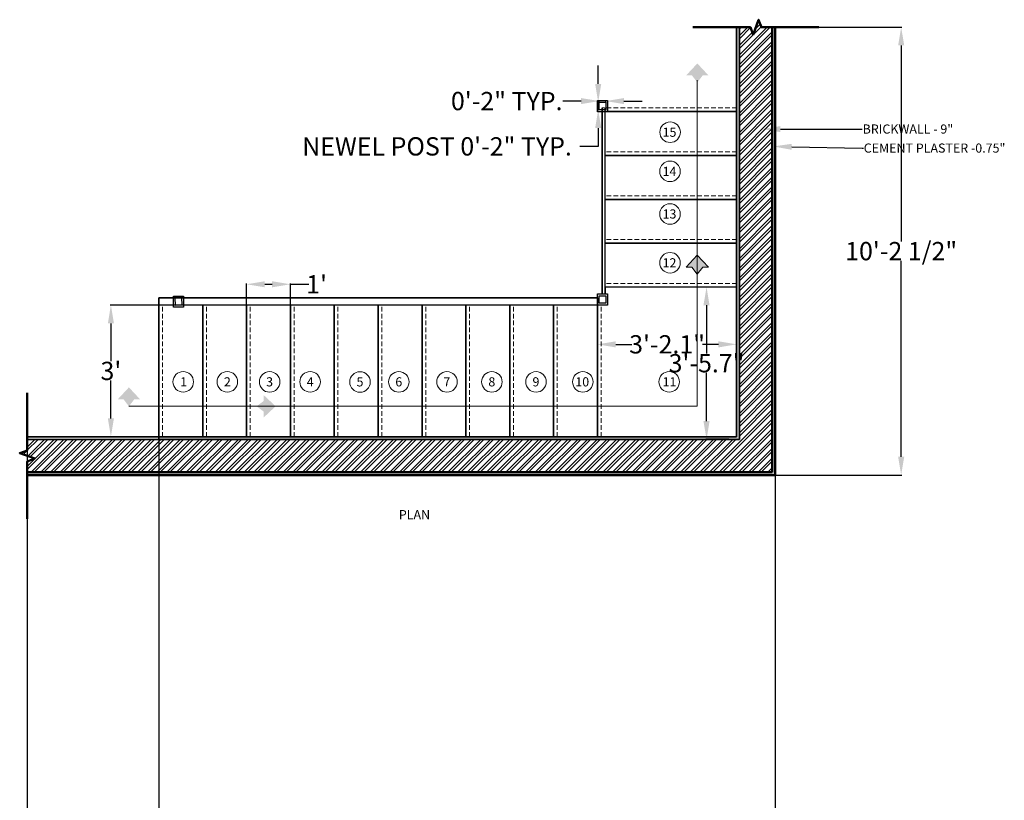
# Model space of a CAD drawing. Units: inches. Extents: x -17 to 288, y -625 to -149.
# Tile 2 of 2: x 18 to 288, y -363 to -149. Entities that reach past the tile are written whole.
import ezdxf
from ezdxf import colors
from ezdxf.entities.mleader import LeaderData, LeaderLine
from ezdxf.math import Vec2, Vec3

# ---------------------------------------------------------------- set-up
doc = ezdxf.new("R2010")
doc.units = ezdxf.units.IN
doc.header["$MEASUREMENT"] = 0
doc.linetypes.add('HIDDEN', pattern=[9.525, 6.35, -3.175])
for name, color, linetype, lineweight in [('A-ANNO-DIMS', 2, 'Continuous', 18), ('A-ANNO-SYMB', 3, 'Continuous', 18), ('A-ANNO-TEXT', 7, 'Continuous', 18), ('A-FLOR-HRAL', 4, 'Continuous', 25), ('A-FLOR-STRS', 1, 'Continuous', 35), ('A-FLOR-STRS-HIDN', 8, 'HIDDEN', 18), ('A-WALL', 7, 'Continuous', 50), ('A-WALL-PATT', 8, 'Continuous', 18)]:
    doc.layers.add(name, color=color, linetype=linetype, lineweight=lineweight)
doc.styles.get("Standard").update_dxf_attribs({"font": 'arial.ttf'})
doc.dimstyles.get("Standard").update_dxf_attribs({"dimtxt": 5, "dimasz": 5, "dimexe": 0.18, "dimexo": 0.0625, "dimgap": 0.09, "dimtad": 0, "dimtih": 1, "dimtoh": 1, "dimdec": 1, "dimzin": 0, "dimdsep": 46, "dimlunit": 3, "dimtxsty": 'Standard', "dimcen": 0, "dimadec": 0, "dimazin": 0, "dimtfac": 1, "dimtdec": 1, "dimtofl": 0, "dimtmove": 0, "dimatfit": 3, "dimfxl": 1, "dimtolj": 1, "dimtzin": 0, "dimarcsym": 1})

# ---------------------------------------------------------------- blocks, each defined once
blk = doc.blocks.new('*D2')
at = {"layer": 'A-ANNO-DIMS', "color": 0, "lineweight": -2, "transparency": 16777216}
for p, q in [((56.28, -227), (43.05, -227)), ((43.23, -232), (43.23, -242.35)), ((43.23, -258), (43.23, -247.64)), ((56.28, -263), (43.05, -263))]:
    blk.add_line(p, q, dxfattribs=at)
at = {"layer": 'A-ANNO-DIMS', "color": 0, "transparency": 16777216}
for points in [[(42.4, -232), (44.07, -232), (43.23, -227)], [(42.4, -258), (44.07, -258), (43.23, -263)]]:
    blk.add_solid(points, dxfattribs=at)
at = {"layer": 'Defpoints', "color": 0, "transparency": 16777216}
for p in [(56.34, -227), (43.23, -263), (56.34, -263)]:
    blk.add_point(p, dxfattribs=at)
at = {"layer": 'A-ANNO-DIMS', "color": 0, "transparency": 16777216, "insert": (43.23, -245), "char_height": 5, "attachment_point": 5}
blk.add_mtext("\\A1;3'", dxfattribs=at)
blk = doc.blocks.new('*D3')
at = {"layer": 'A-ANNO-DIMS', "color": 0, "lineweight": -2, "transparency": 16777216}
for p, q in [((80.34, -226.93), (80.34, -221.11)), ((85.34, -221.29), (87.34, -221.29)), ((92.34, -226.93), (92.34, -221.11)), ((92.34, -221.29), (97.34, -221.29))]:
    blk.add_line(p, q, dxfattribs=at)
at = {"layer": 'A-ANNO-DIMS', "color": 0, "transparency": 16777216}
for points in [[(85.34, -220.46), (85.34, -222.12), (80.34, -221.29)], [(87.34, -220.46), (87.34, -222.12), (92.34, -221.29)]]:
    blk.add_solid(points, dxfattribs=at)
at = {"layer": 'Defpoints', "color": 0, "transparency": 16777216}
for p in [(92.34, -221.29), (80.34, -227), (92.34, -227)]:
    blk.add_point(p, dxfattribs=at)
at = {"layer": 'A-ANNO-DIMS', "color": 0, "transparency": 16777216, "insert": (99.5, -221.29), "char_height": 5, "attachment_point": 5}
blk.add_mtext("\\A1;1'", dxfattribs=at)
blk = doc.blocks.new('*D5')
at = {"layer": 'A-ANNO-DIMS', "color": 0, "lineweight": -2, "transparency": 16777216}
for p, q in [((176.34, -237.39), (176.34, -237.91)), ((181.34, -237.73), (185.73, -237.73)), ((209.41, -237.73), (205.03, -237.73)), ((214.41, -237.39), (214.41, -237.91))]:
    blk.add_line(p, q, dxfattribs=at)
at = {"layer": 'A-ANNO-DIMS', "color": 0, "transparency": 16777216}
for points in [[(181.34, -236.9), (181.34, -238.57), (176.34, -237.73)], [(209.41, -236.9), (209.41, -238.57), (214.41, -237.73)]]:
    blk.add_solid(points, dxfattribs=at)
at = {"layer": 'Defpoints', "color": 0, "transparency": 16777216}
for p in [(176.34, -237.33), (214.41, -237.33), (214.41, -237.73)]:
    blk.add_point(p, dxfattribs=at)
at = {"layer": 'A-ANNO-DIMS', "color": 0, "transparency": 16777216, "insert": (195.38, -237.73), "char_height": 5, "attachment_point": 5}
blk.add_mtext('\\A1;3\'-2.1"', dxfattribs=at)
blk = doc.blocks.new('*D6')
at = {"layer": 'A-ANNO-DIMS', "color": 0, "lineweight": -2, "transparency": 16777216}
for p, q in [((211.19, -222.05), (205.99, -222.05)), ((206.17, -227.05), (206.17, -240.24)), ((206.17, -258.72), (206.17, -245.53)), ((212.26, -263.72), (205.99, -263.72))]:
    blk.add_line(p, q, dxfattribs=at)
at = {"layer": 'A-ANNO-DIMS', "color": 0, "transparency": 16777216}
for points in [[(205.33, -227.05), (207, -227.05), (206.17, -222.05)], [(205.33, -258.72), (207, -258.72), (206.17, -263.72)]]:
    blk.add_solid(points, dxfattribs=at)
at = {"layer": 'Defpoints', "color": 0, "transparency": 16777216}
for p in [(211.26, -222.05), (206.17, -263.72), (212.33, -263.72)]:
    blk.add_point(p, dxfattribs=at)
at = {"layer": 'A-ANNO-DIMS', "color": 0, "transparency": 16777216, "insert": (206.17, -242.89), "char_height": 5, "attachment_point": 5}
blk.add_mtext('\\A1;3\'-5.7"', dxfattribs=at)
blk = doc.blocks.new('NEWEL-POST')
for p, q in [((0, 2.09), (1.75, 2.09)), ((0, 0), (0, 2.09)), ((1.75, 2.09), (1.75, 0)), ((1.75, 0), (0, 0))]:
    blk.add_line(p, q)
blk = doc.blocks.new('*D8')
at = {"layer": 'A-ANNO-DIMS', "color": 0, "lineweight": -2, "transparency": 16777216}
for p, q in [((176.53, -166.47), (176.53, -161.47)), ((176.78, -171.47), (176.35, -171.47)), ((176.78, -173.56), (176.35, -173.56)), ((176.53, -178.56), (176.53, -183.56)), ((176.53, -183.56), (171.53, -183.56))]:
    blk.add_line(p, q, dxfattribs=at)
at = {"layer": 'A-ANNO-DIMS', "color": 0, "transparency": 16777216}
for points in [[(175.7, -166.47), (177.36, -166.47), (176.53, -171.47)], [(175.7, -178.56), (177.36, -178.56), (176.53, -173.56)]]:
    blk.add_solid(points, dxfattribs=at)
at = {"layer": 'Defpoints', "color": 0, "transparency": 16777216}
for p in [(176.84, -171.47), (176.53, -173.56), (176.84, -173.56)]:
    blk.add_point(p, dxfattribs=at)
at = {"layer": 'A-ANNO-DIMS', "color": 0, "transparency": 16777216, "insert": (132.45, -183.56), "char_height": 5, "attachment_point": 5}
blk.add_mtext('\\A1;NEWEL POST 0\'-2" TYP.', dxfattribs=at)
blk = doc.blocks.new('*D9')
at = {"layer": 'A-ANNO-DIMS', "color": 0, "lineweight": -2, "transparency": 16777216}
for p, q in [((171.84, -171.16), (166.84, -171.16)), ((176.84, -171.41), (176.84, -170.98)), ((178.59, -171.41), (178.59, -170.98)), ((183.59, -171.16), (188.59, -171.16))]:
    blk.add_line(p, q, dxfattribs=at)
at = {"layer": 'A-ANNO-DIMS', "color": 0, "transparency": 16777216}
for points in [[(171.84, -170.33), (171.84, -171.99), (176.84, -171.16)], [(183.59, -170.33), (183.59, -171.99), (178.59, -171.16)]]:
    blk.add_solid(points, dxfattribs=at)
at = {"layer": 'Defpoints', "color": 0, "transparency": 16777216}
for p in [(176.84, -171.16), (176.84, -171.47), (178.59, -171.47)]:
    blk.add_point(p, dxfattribs=at)
at = {"layer": 'A-ANNO-DIMS', "color": 0, "transparency": 16777216, "insert": (151.51, -171.16), "char_height": 5, "attachment_point": 5}
blk.add_mtext('\\A1;0\'-2" TYP.', dxfattribs=at)
blk = doc.blocks.new('*D10')
at = {"layer": 'A-ANNO-DIMS', "color": 0, "lineweight": -2, "transparency": 16777216}
for p, q in [((20.34, -273.56), (20.34, -617.82)), ((224.91, -273.56), (224.91, -617.82)), ((25.34, -617.64), (108.36, -617.64)), ((219.91, -617.64), (136.9, -617.64))]:
    blk.add_line(p, q, dxfattribs=at)
at = {"layer": 'A-ANNO-DIMS', "color": 0, "transparency": 16777216}
for points in [[(25.34, -616.81), (25.34, -618.47), (20.34, -617.64)], [(219.91, -616.81), (219.91, -618.47), (224.91, -617.64)]]:
    blk.add_solid(points, dxfattribs=at)
at = {"layer": 'Defpoints', "color": 0, "transparency": 16777216}
for p in [(20.34, -273.5), (224.91, -273.5), (224.91, -617.64)]:
    blk.add_point(p, dxfattribs=at)
at = {"layer": 'A-ANNO-DIMS', "color": 0, "transparency": 16777216, "insert": (122.63, -617.64), "char_height": 5, "attachment_point": 5}
blk.add_mtext('\\A1;17\'-0 1/2"', dxfattribs=at)
blk = doc.blocks.new('*D11')
at = {"layer": 'A-ANNO-DIMS', "color": 0, "lineweight": -2, "transparency": 16777216}
for p, q in [((224.94, -150.95), (259.59, -150.95)), ((259.41, -155.95), (259.41, -209.55)), ((259.41, -268.5), (259.41, -214.9)), ((224.98, -273.5), (259.59, -273.5))]:
    blk.add_line(p, q, dxfattribs=at)
at = {"layer": 'A-ANNO-DIMS', "color": 0, "transparency": 16777216}
for points in [[(258.58, -155.95), (260.25, -155.95), (259.41, -150.95)], [(258.58, -268.5), (260.25, -268.5), (259.41, -273.5)]]:
    blk.add_solid(points, dxfattribs=at)
at = {"layer": 'Defpoints', "color": 0, "transparency": 16777216}
for p in [(224.88, -150.95), (259.41, -150.95), (224.91, -273.5)]:
    blk.add_point(p, dxfattribs=at)
at = {"layer": 'A-ANNO-DIMS', "color": 0, "transparency": 16777216, "insert": (259.41, -212.22), "char_height": 5, "attachment_point": 5}
blk.add_mtext('\\A1;10\'-2 1/2"', dxfattribs=at)
blk = doc.blocks.new('*D12')
at = {"layer": 'A-ANNO-DIMS', "color": 0, "lineweight": -2, "transparency": 16777216}
for p, q in [((20.34, -263.06), (20.34, -617.82)), ((56.34, -263.06), (56.34, -617.82)), ((25.34, -617.64), (31.61, -617.64)), ((51.34, -617.64), (45.08, -617.64))]:
    blk.add_line(p, q, dxfattribs=at)
at = {"layer": 'A-ANNO-DIMS', "color": 0, "transparency": 16777216}
for points in [[(25.34, -616.81), (25.34, -618.47), (20.34, -617.64)], [(51.34, -616.81), (51.34, -618.47), (56.34, -617.64)]]:
    blk.add_solid(points, dxfattribs=at)
at = {"layer": 'Defpoints', "color": 0, "transparency": 16777216}
for p in [(20.34, -263), (56.34, -263), (56.34, -617.64)]:
    blk.add_point(p, dxfattribs=at)
at = {"layer": 'A-ANNO-DIMS', "color": 0, "transparency": 16777216, "insert": (38.34, -617.64), "char_height": 5, "attachment_point": 5}
blk.add_mtext('\\A1;3\'-0"', dxfattribs=at)

msp = doc.modelspace()

# ---------------------------------------------------------------- hatches: boundary and pattern name
at = {"layer": 'A-ANNO-SYMB'}
h = msp.add_hatch(color=256, dxfattribs=at)
h.dxf.hatch_style = 1
h.paths.add_polyline_path([(203.65, -160.86), (200.62, -164.11), (202.16, -164.11), (203.65, -166.05)])
h.paths.add_polyline_path([(203.65, -160.86), (203.65, -166.05), (205.14, -164.11), (206.68, -164.11)])
h = msp.add_hatch(color=256, dxfattribs=at)
h.dxf.hatch_style = 1
h.paths.add_polyline_path([(203.65, -213.37), (200.62, -216.61), (202.16, -216.61), (203.65, -218.55)])
h.paths.add_polyline_path([(203.65, -213.37), (203.65, -218.55), (205.14, -216.61), (206.68, -216.61)])
h = msp.add_hatch(color=256, dxfattribs=at)
h.dxf.hatch_style = 1
h.paths.add_polyline_path([(48.16, -249.5), (45.13, -252.75), (46.67, -252.75), (48.16, -254.69)])
h.paths.add_polyline_path([(48.16, -249.5), (48.16, -254.69), (49.65, -252.75), (51.19, -252.75)])
h = msp.add_hatch(color=256, dxfattribs=at)
h.dxf.hatch_style = 1
h.paths.add_polyline_path([(88.3, -254.68), (85.06, -251.65), (85.06, -253.19), (83.11, -254.68)])
h.paths.add_polyline_path([(88.3, -254.68), (83.11, -254.68), (85.06, -256.17), (85.06, -257.71)])
at = {"layer": 'A-FLOR-STRS'}
h = msp.add_hatch(dxfattribs=at)
h.set_pattern_fill('AR-CONC', color=256, scale=0.2)
h.set_pattern_definition([(50, (-200.1796, -74.3096), (1.4345204, -0.1255043), [0.15, -1.65]), (355, (-200.1796, -74.3096), (-0.2775027, 1.5043843), [0.12, -1.32]), (100.45144, (-200.06, -74.32), (1.1570177, 1.37888), [0.1274804, -1.4022842]), (46.1842, (-200.1796, -73.9096), (2.1344827, -0.3310386), [0.225, -2.475]), (96.63564, (-200.0017, -73.9372), (1.869324, 1.948237), [0.191221, -2.1034275]), (351.18416, (-200.1796, -73.9096), (1.869324, 1.948237), [0.18, -1.98]), (21, (-199.9796, -74.0096), (1.1938141, -0.8052378), [0.15, -1.65]), (326, (-199.9796, -74.0096), (0.4866307, 1.4503), [0.12, -1.32]), (71.45144, (-199.8801, -74.0767), (1.6804448, 0.6450623), [0.1274804, -1.4022842]), (37.5, (-200.1796, -74.3096), (0.0243197, 0.6657877), [0, -1.304, 0, -1.34, 0, -1.325]), (7.5, (-200.1796, -74.3096), (0.5261391, 0.7888234), [0, -0.764, 0, -1.274, 0, -0.505]), (327.5, (-200.6256, -74.3096), (1.06764487, -0.04510974), [0, -0.5, 0, -1.56, 0, -2.07]), (317.5, (-200.8256, -74.3096), (1.1663723, 0.20021), [0, -0.65, 0, -1.036, 0, -1.47])])
h.paths.add_polyline_path([(224.91, -178.83), (224.16, -178.83), (224.16, -272.75), (20.34, -272.75), (20.34, -273.5), (224.91, -273.5)])
h.paths.add_polyline_path([(224.91, -173.05), (224.91, -150.95), (224.16, -150.95), (224.16, -173.05), (224.16, -178.83), (224.91, -178.83)])
h.paths.add_polyline_path([(215.16, -173.05), (215.16, -150.95), (214.41, -150.95), (214.41, -173.05), (214.41, -263), (56.34, -263), (56.34, -263.75), (215.16, -263.75), (215.16, -263)])
h.paths.add_polyline_path([(180.87, -521.9), (214.41, -521.9), (214.41, -521.15), (180.64, -521.15), (68.34, -595.08), (68.34, -595.14), (69.62, -595.14)])
at = {"layer": 'A-WALL-PATT'}
h = msp.add_hatch(dxfattribs=at)
h.set_pattern_fill('ANSI32', color=256, scale=5)
h.set_pattern_definition([(45, (-200.1796, -372.3348), (-1.325825, 1.325825), []), (45, (-199.2957, -372.3348), (-1.325825, 1.325825), [])])
h.paths.add_polyline_path([(224.16, -173.05), (224.16, -150.95), (221.16, -150.95), (220.41, -148.89), (218.91, -153.01), (218.16, -150.95), (215.16, -150.95), (215.16, -173.05), (215.16, -263.75), (56.34, -263.75), (20.34, -263.75), (20.34, -266.75), (18.28, -267.5), (22.4, -269), (20.34, -269.75), (20.34, -272.75), (224.16, -272.75)])

# ---------------------------------------------------------------- linework, layer by layer
at = {"layer": 'A-ANNO-SYMB'}
for p, q in [((203.65, -165.46), (203.65, -254.68)), ((203.65, -213.37), (200.62, -216.61)), ((203.65, -213.37), (206.68, -216.61)), ((200.62, -216.61), (202.16, -216.61)), ((202.16, -216.61), (203.65, -218.55)), ((205.14, -216.61), (203.65, -218.55)), ((206.68, -216.61), (205.14, -216.61)), ((48.16, -254.68), (203.65, -254.68))]:
    msp.add_line(p, q, dxfattribs=at)
for centre in [(196.2, -179.69), (196.18, -190.39), (196.19, -202.07), (196.18, -215.41), (63.02, -247.99), (75.08, -247.99), (86.65, -248.01), (97.72, -247.99), (111.39, -248.03), (122, -248.01), (135.17, -248.01), (147.45, -248.01), (159.53, -248.01), (172.33, -248.01), (195.95, -247.99)]:
    msp.add_circle(centre, 2.81, dxfattribs=at)
at = {"layer": 'A-FLOR-HRAL'}
for p, q in [((176.34, -174.06), (176.34, -170.97)), ((176.34, -170.97), (179.09, -170.97)), ((176.34, -170.97), (176.34, -174.06)), ((179.09, -170.97), (179.09, -174.06)), ((179.09, -174.06), (176.34, -174.06)), ((178.41, -223.9), (178.41, -173.05)), ((214.41, -222.05), (178.41, -222.05)), ((178.41, -222.05), (178.41, -223.9)), ((60.34, -227.6), (60.34, -224.51)), ((60.34, -224.51), (63.09, -224.51)), ((63.09, -224.51), (63.09, -227.6)), ((176.34, -227), (176.34, -223.9)), ((176.34, -223.9), (179.09, -223.9)), ((179.09, -223.9), (179.09, -227)), ((179.09, -227), (56.34, -227)), ((63.09, -227.6), (60.34, -227.6))]:
    msp.add_line(p, q, dxfattribs=at)
at = {"layer": 'A-FLOR-STRS'}
for p, q in [((214.41, -173.05), (214.41, -150.95)), ((214.41, -150.95), (215.16, -150.95)), ((215.16, -173.05), (215.16, -150.95)), ((177.66, -223.9), (177.66, -173.05)), ((214.41, -174.05), (178.41, -174.05)), ((214.41, -263), (214.41, -173.05)), ((215.16, -263.75), (215.16, -173.05)), ((214.41, -186.05), (178.41, -186.05)), ((214.41, -198.05), (178.41, -198.05)), ((214.41, -210.05), (178.41, -210.05)), ((176.34, -225), (56.34, -225)), ((56.34, -263.75), (56.34, -225)), ((176.34, -263), (176.34, -225)), ((68.34, -263), (68.34, -227)), ((80.34, -263), (80.34, -227)), ((92.34, -263), (92.34, -227)), ((104.34, -263), (104.34, -227)), ((116.34, -263), (116.34, -227)), ((128.34, -263), (128.34, -227)), ((140.34, -263), (140.34, -227)), ((152.34, -263), (152.34, -227)), ((164.34, -263), (164.34, -227)), ((56.34, -263), (20.34, -263)), ((20.34, -263), (20.34, -263.75)), ((56.34, -263.75), (20.34, -263.75)), ((56.34, -263), (214.41, -263)), ((56.34, -263.75), (215.16, -263.75)), ((215.16, -263.75), (215.16, -263))]:
    msp.add_line(p, q, dxfattribs=at)
at = {"layer": 'A-FLOR-STRS-HIDN', "ltscale": 0.2}
for p, q in [((214.41, -173.05), (177.66, -173.05)), ((214.41, -185.05), (178.41, -185.05)), ((214.41, -197.05), (178.41, -197.05)), ((214.41, -209.05), (178.41, -209.05)), ((214.41, -221.05), (178.41, -221.05)), ((57.34, -263), (57.34, -227)), ((69.34, -263), (69.34, -227)), ((81.34, -263), (81.34, -227)), ((93.34, -263), (93.34, -227)), ((105.34, -263), (105.34, -227)), ((117.34, -263), (117.34, -227)), ((129.34, -263), (129.34, -227)), ((141.34, -263), (141.34, -227)), ((153.34, -263), (153.34, -227)), ((165.34, -263), (165.34, -227)), ((177.34, -263), (177.34, -227))]:
    msp.add_line(p, q, dxfattribs=at)
at = {"layer": 'A-WALL'}
for p, q in [((224.16, -173.05), (224.16, -150.95)), ((224.16, -150.95), (224.88, -150.95)), ((224.88, -150.95), (224.91, -150.95)), ((224.91, -173.05), (224.91, -150.95)), ((224.16, -272.75), (224.16, -173.05)), ((224.91, -273.5), (224.91, -173.05)), ((224.16, -272.75), (20.34, -272.75)), ((20.34, -272.75), (20.34, -273.5)), ((176.34, -273.5), (20.34, -273.5)), ((224.91, -273.5), (20.34, -273.5))]:
    msp.add_line(p, q, dxfattribs=at)
for points in [[(202.41, -150.95), (218.16, -150.95), (218.91, -153.01), (220.41, -148.89), (221.16, -150.95), (236.91, -150.95)], [(20.34, -251), (20.34, -266.75), (18.28, -267.5), (22.4, -269), (20.34, -269.75), (20.34, -285.5)]]:
    msp.add_lwpolyline(points, dxfattribs=at)

# ---------------------------------------------------------------- block references
at = {"layer": 'A-FLOR-HRAL'}
for p, rotation in [((178.59, -171.47), 180), ((62.57, -224.93), 181.2726933592207)]:
    msp.add_blockref('NEWEL-POST', p, dxfattribs=dict(at, rotation=rotation))
msp.add_blockref('NEWEL-POST', (176.84, -226.5), dxfattribs=at)

# ---------------------------------------------------------------- texts
at = {"layer": 'A-ANNO-TEXT'}
for s, p in [('15', (194.14, -180.93)), ('14', (194.14, -191.65)), ('13', (194.14, -203.3)), ('12', (194.14, -216.67)), ('1', (62.17, -249.24)), ('2', (74.15, -249.24)), ('3', (85.69, -249.24)), ('4', (96.81, -249.24)), ('5', (110.42, -249.24)), ('6', (121.04, -249.24)), ('7', (134.19, -249.24)), ('8', (146.49, -249.24)), ('9', (158.56, -249.24)), ('10', (170.28, -249.24)), ('11', (194.14, -249.24))]:
    msp.add_text(s, height=2.5, dxfattribs=at).set_placement(p)
at = {"layer": 'A-ANNO-TEXT', "insert": (122, -283.08), "char_height": 2.5, "attachment_point": 1}
msp.add_mtext_dynamic_manual_height_columns('PLAN', width=63.442, gutter_width=12.5, heights=[0], dxfattribs=at)

# ---------------------------------------------------------------- dimensions: what is measured, and where the dimension line sits
at = {"layer": 'A-ANNO-DIMS'}
for base, p1, p2, override, picture, middle in [((259.415, -150.9491), (224.915, -273.4952), (224.8771, -150.9491), {"dimdec": 1, "dimlfac": 1, "dimrnd": 0, "dimzin": 1, "dimdsep": 46, "dimlunit": 4, "dimfrac": 2}, '*D11', (259.415, -212.2221)), ((206.17, -263.72), (211.26, -222.05), (212.33, -263.72), {"dimclrd": 0, "dimclre": 0, "dimclrt": 0}, '*D6', (206.17, -242.89)), ((43.23, -263), (56.34, -227), (56.34, -263), {"dimclrd": 0, "dimclre": 0, "dimclrt": 0}, '*D2', (43.23, -245))]:
    dim = msp.add_linear_dim(base=base, p1=p1, p2=p2, angle=90, dimstyle='Standard', override=override, dxfattribs=at)
    dim.commit()
    dim.dimension.update_dxf_attribs({"geometry": picture, "text_midpoint": middle})
for base, p1, p2, angle, text, picture, middle in [((176.53, -173.56), (176.84, -171.47), (176.84, -173.56), 270, 'NEWEL POST <> TYP.', '*D8', (132.45, -183.56)), ((176.8436, -171.1585), (178.5944, -171.4723), (176.8436, -171.4723), 180, '<> TYP.', '*D9', (151.5149, -171.1585))]:
    dim = msp.add_linear_dim(base=base, p1=p1, p2=p2, angle=angle, text=text, dimstyle='Standard', override={"dimdec": 1, "dimrnd": 0, "dimzin": 1, "dimlunit": 4, "dimfrac": 2}, dxfattribs=at)
    dim.commit()
    dim.dimension.update_dxf_attribs({"geometry": picture, "text_midpoint": middle})
for base, p1, p2, override, picture, middle in [((92.34, -221.29), (80.34, -227), (92.34, -227), {"dimclrd": 0, "dimclre": 0, "dimclrt": 0}, '*D3', (99.5, -221.29)), ((214.41, -237.73), (176.34, -237.33), (214.41, -237.33), {"dimclrd": 0, "dimclre": 0, "dimclrt": 0}, '*D5', (195.38, -237.73)), ((56.34, -617.64), (20.34, -263), (56.34, -263), {"dimdec": 1, "dimlfac": 1, "dimrnd": 0, "dimzin": 1, "dimdsep": 46, "dimlunit": 4, "dimfrac": 2}, '*D12', (38.34, -617.64)), ((224.91, -617.64), (20.34, -273.5), (224.91, -273.5), {"dimdec": 1, "dimlfac": 1, "dimrnd": 0, "dimzin": 1, "dimdsep": 46, "dimlunit": 4, "dimfrac": 2}, '*D10', (122.63, -617.64))]:
    dim = msp.add_linear_dim(base=base, p1=p1, p2=p2, dimstyle='Standard', override=override, dxfattribs=at)
    dim.commit()
    dim.dimension.update_dxf_attribs({"geometry": picture, "text_midpoint": middle})

# ---------------------------------------------------------------- leaders
at = {"layer": 'A-ANNO-SYMB'}
ml = msp.add_multileader_mtext('Standard', dxfattribs=at)
ml.set_content('BRICKWALL - 9"', color=256)
ml.set_leader_properties()
ml.build(insert=Vec2(0, 0))
ml.multileader.update_dxf_attribs({"dogleg_length": 0.36, "arrow_head_size": 5})
ctx = ml.context
ctx.base_point, ctx.char_height, ctx.arrow_head_size, ctx.landing_gap_size, ctx.plane_origin = Vec3(248.78, -178.83), 2.5, 5, 0.09, Vec3(221.36, -178.83)
notes = []
notes.append((ctx, [(0, (1, 1, 0), (248.42, -178.83), (1, 0), 0.36, [(0, [(221.36, -178.83)], 0, [])])]))
ctx.mtext.insert, ctx.mtext.flow_direction = Vec3(248.87, -177.56), 5
ml = msp.add_multileader_mtext('Standard', dxfattribs=at)
ml.set_content('CEMENT PLASTER -0.75"', color=256)
ml.set_leader_properties()
ml.build(insert=Vec2(0, 0))
ml.multileader.update_dxf_attribs({"dogleg_length": 0.36, "arrow_head_size": 5})
ctx = ml.context
ctx.base_point, ctx.char_height, ctx.arrow_head_size, ctx.landing_gap_size, ctx.plane_origin = Vec3(249.08, -184.04), 2.5, 5, 0.09, Vec3(224.48, -183.58)
notes.append((ctx, [(0, (1, 1, 0), (248.72, -184.04), (1, 0), 0.36, [(0, [(224.48, -183.58)], 0, [])])]))
ctx.mtext.insert, ctx.mtext.flow_direction = Vec3(249.17, -182.77), 5
for ctx, leaders in notes:
    for number, flags, end, landing, length, lines in leaders:
        leader = LeaderData()
        leader.index, (leader.has_last_leader_line, leader.has_dogleg_vector, leader.attachment_direction) = number, flags
        leader.last_leader_point, leader.dogleg_vector, leader.dogleg_length = Vec3(end), Vec3(landing), length
        for number, points, colour, breaks in lines:
            line = LeaderLine()
            line.index, line.vertices, line.color, line.breaks = number, Vec3.list(points), colors.encode_raw_color(colour), breaks
            leader.lines.append(line)
        ctx.leaders.append(leader)

doc.saveas('drawing.dxf')
